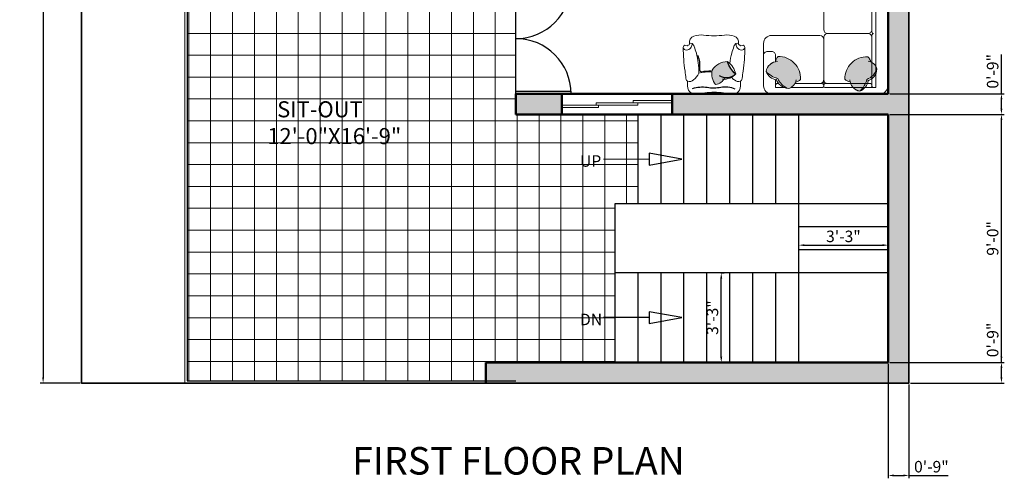
# Model space of a CAD drawing. Units: inches. Extents: x 1734 to 4011, y 1071 to 1891.
# Tile 10 of 27: x 2226 to 2654, y 1083 to 1282. Entities that reach past the tile are written whole.
import ezdxf

# ---------------------------------------------------------------- set-up
doc = ezdxf.new("R2010")
doc.units = ezdxf.units.IN
for name, color, linetype, lineweight in [('A-ANNO-DIMS', 2, 'Continuous', 18), ('A-ANNO-TEXT', 7, 'Continuous', 25), ('A-AREA-IDEN', 3, 'Continuous', 18), ('A-DOOR', 3, 'Continuous', 25), ('A-FLOR-OTLN', 7, 'Continuous', 25), ('A-FLOR-PATT', 252, 'Continuous', 13), ('A-FLOR-STRS', 2, 'Continuous', 25), ('A-FURN', 8, 'Continuous', 18), ('A-FURN-PATT', 252, 'Continuous', 13), ('A-GLAZ', 4, 'Continuous', 18), ('A-WALL', 7, 'Continuous', 50), ('A-WALL-PATT', 8, 'Continuous', 13), ('C-PROP', 1, 'Continuous', 35)]:
    doc.layers.add(name, color=color, linetype=linetype, lineweight=lineweight)
doc.layers.add('IFF-FURN-DETAIL', color=250, linetype='Continuous')
doc.styles.get("Standard").update_dxf_attribs({"font": 'arial.ttf'})
doc.dimstyles.new('ISO-25', dxfattribs={"dimtxt": 5, "dimasz": 2.5, "dimexe": 1.25, "dimexo": 0.625, "dimtad": 1, "dimdec": 1, "dimlunit": 3, "dimtxsty": 'Standard', "dimcen": 2.5, "dimclrt": 1, "dimadec": 0, "dimazin": 0, "dimtfac": 1, "dimtdec": 1, "dimtmove": 0, "dimatfit": 3, "dimfxl": 1, "dimarcsym": 0})

# ---------------------------------------------------------------- blocks, each defined once
blk = doc.blocks.new('*D17')
at = {"layer": 'A-ANNO-DIMS', "color": 0, "lineweight": -2, "transparency": 16777216}
for p, q in [((2251.86, 1844.06), (2234.55, 1844.06)), ((2235.8, 1841.56), (2235.8, 1126.56)), ((2251.86, 1124.06), (2234.55, 1124.06))]:
    blk.add_line(p, q, dxfattribs=at)
at = {"layer": 'A-ANNO-DIMS', "color": 0, "transparency": 16777216}
for points in [[(2235.38, 1841.56), (2236.21, 1841.56), (2235.8, 1844.06)], [(2235.38, 1126.56), (2236.21, 1126.56), (2235.8, 1124.06)]]:
    blk.add_solid(points, dxfattribs=at)
at = {"layer": 'Defpoints', "color": 0, "transparency": 16777216}
for p in [(2252.48, 1844.06), (2235.8, 1124.06), (2252.48, 1124.06)]:
    blk.add_point(p, dxfattribs=at)
at = {"layer": 'A-ANNO-DIMS', "color": 0, "transparency": 16777216, "insert": (2230.58, 1484.06), "char_height": 5, "attachment_point": 5, "rotation": 90}
blk.add_mtext("{\\H1.8x;60'}", dxfattribs=at)
blk = doc.blocks.new('*D18')
at = {"layer": 'A-ANNO-DIMS', "color": 0, "lineweight": -2, "transparency": 16777216}
for p, q in [((2530.68, 1172.06), (2532.08, 1172.06)), ((2530.83, 1135.56), (2530.83, 1169.56)), ((2530.68, 1133.06), (2532.08, 1133.06))]:
    blk.add_line(p, q, dxfattribs=at)
at = {"layer": 'A-ANNO-DIMS', "color": 0, "transparency": 16777216}
for points in [[(2530.41, 1169.56), (2531.25, 1169.56), (2530.83, 1172.06)], [(2530.41, 1135.56), (2531.25, 1135.56), (2530.83, 1133.06)]]:
    blk.add_solid(points, dxfattribs=at)
at = {"layer": 'Defpoints', "color": 0, "transparency": 16777216}
for p in [(2530.05, 1172.06), (2530.83, 1172.06), (2530.05, 1133.06)]:
    blk.add_point(p, dxfattribs=at)
at = {"layer": 'A-ANNO-DIMS', "color": 0, "transparency": 16777216, "insert": (2527.65, 1152.56), "char_height": 5, "attachment_point": 5, "rotation": 90}
blk.add_mtext('3\'-3"', dxfattribs=at)
blk = doc.blocks.new('*D19')
at = {"layer": 'A-ANNO-DIMS', "color": 0, "lineweight": -2, "transparency": 16777216}
for p, q in [((2564.48, 1186.44), (2564.48, 1182.86)), ((2566.98, 1184.11), (2600.98, 1184.11)), ((2603.48, 1186.44), (2603.48, 1182.86))]:
    blk.add_line(p, q, dxfattribs=at)
at = {"layer": 'A-ANNO-DIMS', "color": 0, "transparency": 16777216}
for points in [[(2566.98, 1184.52), (2566.98, 1183.69), (2564.48, 1184.11)], [(2600.98, 1184.52), (2600.98, 1183.69), (2603.48, 1184.11)]]:
    blk.add_solid(points, dxfattribs=at)
at = {"layer": 'Defpoints', "color": 0, "transparency": 16777216}
for p in [(2564.48, 1187.06), (2603.48, 1187.06), (2603.48, 1184.11)]:
    blk.add_point(p, dxfattribs=at)
at = {"layer": 'A-ANNO-DIMS', "color": 0, "transparency": 16777216, "insert": (2583.98, 1187.29), "char_height": 5, "attachment_point": 5}
blk.add_mtext('3\'-3"', dxfattribs=at)
blk = doc.blocks.new("MD D 4'")
for p, q in [((0, 24), (0, 0)), ((1, 24), (1, 0)), ((47, 24), (47, 0)), ((48, 24), (48, 0)), ((0, 0), (1, 0)), ((48, 0), (47, 0))]:
    blk.add_line(p, q)
for centre, start, end in [((0, 0), 0, 90), ((48, 0), 90, 180)]:
    blk.add_arc(centre, 24, start, end)
blk = doc.blocks.new('SOFA 1')
at = {"transparency": 33554687}
h = blk.add_hatch(color=256, dxfattribs=at)
h.dxf.hatch_style = 1
h.paths.add_polyline_path([(3723.52, 1308.63, 0.147724), (3717.76, 1305.24, 0.310469), (3722.42, 1300.4), (3722.42, 1300.25, 0.156703), (3723.62, 1297.8, 0.425821), (3734.69, 1309.08, 0.121928), (3732.05, 1310.63, 0.233216), (3728.6, 1313.59, 0.213835)])
h = blk.add_hatch(color=256, dxfattribs=at)
h.dxf.hatch_style = 1
h.paths.add_polyline_path([(3769.65, 1307.6, 0.084911), (3767.15, 1309.12, 0.046133), (3766.46, 1311.13), (3759.18, 1311.13, 0.039409), (3758.92, 1310.24, 0.165523), (3756.31, 1309.02, 0.42585), (3767.59, 1297.95, 0.121928), (3769.15, 1300.58, 0.027403), (3769.65, 1300.83)])
h.paths.add_polyline_path([(3765.34, 1313.08), (3760.4, 1313.08, 0.097704), (3759.18, 1311.13), (3766.46, 1311.13, 0.04873)])
h.paths.add_polyline_path([(3763.76, 1314.88, 0.16488), (3760.4, 1313.08), (3765.34, 1313.08, 0.051917)])
h.paths.add_polyline_path([(3771.6, 1305.17, 0.090388), (3769.65, 1307.6), (3769.65, 1300.83, 0.136035), (3771.6, 1302.77)])
h = blk.add_hatch(color=256, dxfattribs=at)
h.dxf.hatch_style = 1
h.paths.add_polyline_path([(3769.16, 1235.96, 0.122267), (3767.6, 1238.61, 0.425972), (3756.32, 1227.54, 0.165563), (3758.93, 1226.32, 0.309481), (3763.76, 1221.69, 0.002677), (3763.83, 1221.72, 0.146094), (3767.16, 1227.43, 0.212433), (3772.1, 1232.48, 0.235342)])
h = blk.add_hatch(color=256, dxfattribs=at)
h.dxf.hatch_style = 1
h.paths.add_polyline_path([(3769.16, 1225.36, 0.122267), (3767.6, 1228.01, 0.425972), (3756.32, 1216.94, 0.165563), (3758.93, 1215.72, 0.309481), (3763.76, 1211.09, 0.002677), (3763.83, 1211.12, 0.146094), (3767.16, 1216.83, 0.212433), (3772.1, 1221.88, 0.235342)])
for p, q in [((3720.45, 1316.13), (3773.58, 1316.13)), ((3777.51, 1312.19), (3777.51, 1213.72))]:
    blk.add_line(p, q, dxfattribs=at)
for points in [[(3717.76, 1305.24, -0.147724), (3723.52, 1308.63, -0.213355), (3728.59, 1313.59, 0.213355), (3723.52, 1308.63, 0.147724), (3717.76, 1305.24, -0.249545), (3722.86, 1309.34, 0.249545), (3717.75, 1305.25, 0.356779), (3723.4, 1300.28, -0.356779), (3717.76, 1305.24)], [(3728.58, 1313.6, -0.306333), (3732.42, 1309.31, 0.306333), (3728.58, 1313.6, 0.306674), (3722.72, 1308.89, -0.306674), (3728.58, 1313.6)], [(3763.76, 1314.88, -0.147724), (3767.15, 1309.12, -0.213355), (3772.1, 1304.05, 0.213355), (3767.15, 1309.12, 0.147724), (3763.76, 1314.88, -0.249545), (3767.86, 1309.77, 0.249545), (3763.77, 1314.89, 0.356779), (3758.8, 1309.23, -0.356779), (3763.76, 1314.88)], [(3734.69, 1309.08, -0.425972), (3723.62, 1297.8, -0.165552), (3722.4, 1300.4, 0.165552), (3723.62, 1297.79, 0.425972), (3734.69, 1309.07, 0.121514), (3732.07, 1310.63, -0.121514), (3734.69, 1309.08)], [(3767.6, 1297.95, -0.425972), (3756.31, 1309.01, -0.165552), (3758.92, 1310.24, 0.165552), (3756.31, 1309.02, 0.425972), (3767.59, 1297.95, 0.121514), (3769.14, 1300.57, -0.121514), (3767.6, 1297.95)], [(3772.11, 1304.06, -0.306333), (3767.83, 1300.22, 0.306333), (3772.11, 1304.06, 0.306674), (3767.4, 1309.91, -0.306674), (3772.11, 1304.06)], [(3770.44, 1286.63, -0.414214), (3769.66, 1287.4, 0.414214), (3770.44, 1286.63, 0.414214), (3769.66, 1285.83, -0.414214), (3770.44, 1286.63)], [(3748.01, 1262.99, -0.414214), (3746.05, 1264.95, 0.414214), (3748.01, 1262.97, 0.414213), (3746.05, 1261.01, -0.414213), (3748.01, 1262.99)], [(3770.44, 1262.99, -0.414214), (3769.66, 1263.77, 0.414214), (3770.44, 1262.99, 0.414214), (3769.66, 1262.19, -0.414214), (3770.44, 1262.99)], [(3770.83, 1262.97, -0.414214), (3771.61, 1262.19, 0.414214), (3770.83, 1262.99, 0.414214), (3771.61, 1263.77, -0.414214), (3770.83, 1262.97)], [(3748.01, 1239.35, -0.414214), (3746.05, 1241.31, 0.414214), (3748.01, 1239.33, 0.414213), (3746.05, 1237.37, -0.414213), (3748.01, 1239.35)], [(3767.7, 1239.33, -0.414214), (3769.66, 1237.37, 0.414214), (3767.7, 1239.35, 0.414214), (3769.66, 1241.31, -0.414214), (3767.7, 1239.33)], [(3756.32, 1227.54, -0.425972), (3767.6, 1238.61, -0.121514), (3769.16, 1235.98, 0.121514), (3767.6, 1238.61, 0.425972), (3756.32, 1227.54, 0.165552), (3758.93, 1226.32, -0.165552), (3756.32, 1227.54)], [(3772.1, 1232.5, -0.306674), (3767.41, 1226.64, 0.306674), (3772.1, 1232.5, 0.306333), (3767.84, 1236.34, -0.306333), (3772.1, 1232.5)], [(3770.44, 1239.35, -0.414214), (3769.66, 1240.13, 0.414214), (3770.44, 1239.33, 0.414214), (3769.66, 1238.55, -0.414214), (3770.44, 1239.35)], [(3770.83, 1239.33, -0.414214), (3771.61, 1238.55, 0.414214), (3770.83, 1239.35, 0.414214), (3771.61, 1240.13, -0.414214), (3770.83, 1239.33)], [(3763.78, 1221.67, 0.249545), (3767.87, 1226.78, -0.249545), (3763.76, 1221.69, -0.356779), (3758.81, 1227.32, 0.356779), (3763.77, 1221.68, 0.147724), (3767.16, 1227.43, 0.213355), (3772.11, 1232.51, -0.213355), (3767.16, 1227.43, -0.147724), (3763.78, 1221.67)], [(3756.32, 1216.94, -0.200233), (3759.49, 1224.76, 0.200233), (3756.32, 1216.94, 0.165552), (3758.93, 1215.72, -0.165552), (3756.32, 1216.94)], [(3772.1, 1221.9, -0.306674), (3767.41, 1216.04, 0.306674), (3772.1, 1221.9, -0.213355), (3767.16, 1216.83, -0.147724), (3763.77, 1211.08, 0.147724), (3767.15, 1216.83, 0.213355), (3772.1, 1221.9)], [(3763.76, 1211.09, -0.356779), (3758.81, 1216.72, 0.356779), (3763.76, 1211.09, 0.249545), (3767.87, 1216.18, -0.249545), (3763.76, 1211.09)]]:
    blk.add_lwpolyline(points, format="xyb", dxfattribs=at)
for points in [[(3722.42, 1313.08), (3722.42, 1309.23), (3722.42, 1313.08), (3726.57, 1313.08)], [(3729.85, 1313.08), (3745.25, 1313.08)], [(3768.11, 1313.08), (3746.78, 1313.08)], [(3771.6, 1313.08), (3767.75, 1313.08), (3771.6, 1313.08), (3771.6, 1308.93)], [(3771.6, 1313.08), (3771.61, 1233.74)], [(3716.51, 1312.2), (3716.51, 1291.44)], [(3723.21, 1311.13), (3723.93, 1311.13)], [(3731.82, 1311.13), (3745.25, 1311.13)], [(3746.01, 1312.3), (3746.01, 1288.55)], [(3746.01, 1310.97), (3746.01, 1311.36)], [(3746.01, 1288.54), (3746.01, 1308.23)], [(3768.87, 1311.13), (3746.78, 1311.13)], [(3769.66, 1287.39), (3769.65, 1312.3)], [(3769.65, 1309.43), (3769.65, 1308.71)], [(3722.42, 1300.39), (3722.42, 1297.33)], [(3720.45, 1295.38), (3718.48, 1295.38)], [(3720.45, 1287.5), (3744.09, 1287.5)], [(3746.02, 1284.63), (3746.02, 1264.94)], [(3747.99, 1286.6), (3767.69, 1286.6)], [(3769.66, 1263.75), (3769.66, 1285.81)], [(3769.66, 1277.18), (3769.66, 1263.75)], [(3746.02, 1260.99), (3746.02, 1241.3)], [(3747.99, 1262.97), (3767.69, 1262.97)], [(3769.66, 1240.12), (3769.66, 1262.18)], [(3770.43, 1262.97), (3770.82, 1262.97)], [(3746.02, 1237.36), (3746.02, 1213.74)], [(3747.99, 1239.33), (3767.69, 1239.33)], [(3769.66, 1235.71), (3769.66, 1238.54)], [(3770.43, 1239.33), (3770.82, 1239.33)], [(3769.66, 1225.11), (3769.66, 1227.82)], [(3771.61, 1223.14), (3771.61, 1230.47)], [(3767.76, 1215.72), (3771.61, 1215.72), (3771.61, 1219.84), (3771.61, 1215.72)], [(3769.66, 1216.5), (3769.66, 1217.22)], [(3753.91, 1211.77), (3753.91, 1213.74)], [(3755.86, 1215.72), (3758.92, 1215.72)], [(3749.97, 1209.8), (3773.58, 1209.8)]]:
    blk.add_lwpolyline(points, close=True, dxfattribs=at)
for points in [[(3770.43, 1313.08, 0.414214), (3769.65, 1312.3, -0.414214)], [(3771.6, 1312.3, 0.414214), (3770.82, 1313.08, -0.414214)], [(3722.42, 1311.91, 0.414214), (3723.2, 1311.13, -0.414214)], [(3716.51, 1297.34, 0.414214), (3718.47, 1295.38, -0.414214)], [(3720.44, 1295.38, 0.414214), (3722.4, 1297.34, -0.414214)], [(3716.51, 1291.45, 0.414212), (3720.44, 1287.52, -0.414212)], [(3746.03, 1288.56, 0.414214), (3747.99, 1286.6, 0.414213), (3746.03, 1284.64, -0.414213), (3747.99, 1286.6, -0.414214)], [(3769.66, 1284.64, 0.414214), (3767.7, 1286.6, 0.414214), (3769.66, 1288.56, -0.414214), (3767.7, 1286.6, -0.414214)], [(3769.66, 1261.01, 0.414214), (3767.7, 1262.97, 0.414214), (3769.66, 1264.93, -0.414214), (3767.7, 1262.97, -0.414214)], [(3769.16, 1225.36, 0.071861), (3768.39, 1227.01, -0.071861)], [(3772.13, 1221.9, 0.306333), (3767.84, 1225.74, -0.306333)], [(3769.66, 1216.52, 0.414214), (3770.44, 1215.74, -0.414214)], [(3770.83, 1215.74, 0.414214), (3771.61, 1216.52, -0.414214)], [(3746.05, 1213.76, 0.414212), (3749.98, 1209.82, -0.414212)], [(3755.87, 1215.72, 0.414214), (3753.91, 1213.76, -0.414214)], [(3755.87, 1209.8, -0.414214), (3753.91, 1211.76, 0.414214)]]:
    blk.add_lwpolyline(points, format="xyb", close=True, dxfattribs=at)
for centre, radius, start, end in [((3720.44, 1312.2), 3.93, 90.0002, 179.9998), ((3720.44, 1312.19), 3.94, 89.9158, 179.9154), ((3745.22, 1312.29), 0.789, 0.8425, 90.8425), ((3746.8, 1312.29), 0.789, 89.1575, 179.1575), ((3768.87, 1312.3), 0.777, 360, 90), ((3773.58, 1312.2), 3.93, 0.0002, 89.9998), ((3773.57, 1312.19), 3.94, 359.9158, 89.9154), ((3744.09, 1309.21), 1.92, 358.766, 90.5111), ((3745.24, 1311.91), 0.777, 270, 0), ((3745.24, 1311.91), 0.777, 270, 0), ((3746.79, 1311.91), 0.777, 180, 270), ((3746.79, 1311.91), 0.777, 180, 270), ((3747.93, 1309.21), 1.92, 89.4889, 181.234), ((3768.87, 1311.91), 0.777, 270, 0), ((3744.08, 1289.48), 1.96, 270, 360), ((3744.08, 1289.48), 1.96, 270, 360), ((3773.58, 1213.73), 3.93, 270.0002, 359.9998), ((3773.59, 1213.73), 3.93, 269.9156, 359.9152)]:
    blk.add_arc(centre, radius, start, end, dxfattribs=at)
blk = doc.blocks.new('PILLOW-1')
at = {"color": 0}
blk.add_lwpolyline([(198, -165, -0.232884), (126, -346, -0.184752), (-44, -234, -0.286563), (75, -22, -0.237978), (273, -68, -0.243587), (179, -195, 4.263709)], format="xyb", dxfattribs=at)
at = {"layer": 'IFF-FURN-DETAIL'}
blk.add_lwpolyline([(148, -118, -0.343333), (126, -342, 0.126408), (-40, -233, -5.969376)], format="xyb", dxfattribs=at)
blk = doc.blocks.new('CLNG90')
for points in [[(689, 370, 0.157831), (677, 385, 0.121013), (646, 395, -0.017334), (547, 407, 0.041496), (215, 431, 0.153531), (191, 423, 0.382906), (185, 395, -0.284047), (184, 361, 0.011997), (177, 351, -0.370479), (160, 345, 0.380647), (56, 282, 0.117468), (41, 146, -0.027775), (50, 0, -8.773898)], [(160, 345, 0.22481), (160, 306, 0.055398), (209, 322, 0.180116), (249, 368, 0.194833), (248, 405, 0.242377), (215, 431, 1.52074)], [(160, 345, 0.22481), (160, 306, 0.055398), (209, 322, 0.180116), (249, 368, 0.194833), (248, 405, 0.242377), (215, 431, 1.52074)], [(689, 370, -0.235486), (671, 286, -0.134038), (574, 215, -0.079303), (293, 248, -0.027048), (199, 280, -0.106276), (160, 306, -1.699)], [(689, 370, -0.235486), (671, 286, -0.134038), (574, 215, -0.079303), (293, 248, -0.027048), (199, 280, -0.106276), (160, 306, -1.699)], [(689, 370, -0.146607), (814, 357, -0.305296), (862, 286, -0.042137), (852, 131, 0.040285), (843, 0, 3.952121)], [(574, 215, 0.061244), (556, 29, 3.376255)], [(574, 215, 0.061244), (556, 29, 3.376255)], [(689, -370, -0.157831), (677, -385, -0.121013), (646, -395, 0.017334), (547, -407, -0.041496), (215, -431, -0.153531), (191, -423, -0.382906), (185, -395, 0.284047), (184, -361, -0.011997), (177, -351, 0.370479), (160, -345, -0.380647), (56, -282, -0.117468), (41, -146, 0.027775), (50, 0, 8.773898)], [(689, -370, 0.146607), (814, -357, 0.305296), (862, -286, 0.042137), (852, -131, -0.040285), (843, 0, -3.952121)], [(437, -220, 0.041086), (293, -248, 0.027048), (199, -280, 0.106276), (160, -306, 1.699)], [(437, -220, 0.041086), (293, -248, 0.027048), (199, -280, 0.106276), (160, -306, 1.699)], [(689, -370, 0.235486), (671, -286, 0.060693), (632, -247, 0.001296)], [(689, -370, 0.235486), (671, -286, 0.060693), (632, -247, 0.001296)], [(160, -345, -0.22481), (160, -306, -0.055398), (209, -322, -0.180116), (249, -368, -0.194833), (248, -405, -0.242377), (215, -431, -1.52074)], [(160, -345, -0.22481), (160, -306, -0.055398), (209, -322, -0.180116), (249, -368, -0.194833), (248, -405, -0.242377), (215, -431, -1.52074)]]:
    blk.add_lwpolyline(points, format="xyb")
at = {"layer": 'IFF-FURN-DETAIL'}
for points in [[(791, 301, 0.124986), (774, 96, -0.091334), (771, -95, 0.164688), (797, -292, 1.068868)], [(791, 301, 0.124986), (774, 96, -0.091334), (771, -95, 0.164688), (797, -292, 1.068868)], [(328, 228, 0.109125), (508, 203, -0.16587), (546, 194, -0.314359), (555, 172, 0.072017), (544, 42, 4.351186)], [(328, 228, 0.109125), (508, 203, -0.16587), (546, 194, -0.314359), (555, 172, 0.072017), (544, 42, 4.351186)]]:
    blk.add_lwpolyline(points, format="xyb", dxfattribs=at)
at = {"xscale": 1.016, "yscale": 1.016, "zscale": 1.016}
blk.add_blockref('PILLOW-1', (458, 47), dxfattribs=at)
blk.add_blockref('PILLOW-1', (458, 47), dxfattribs=at)
blk = doc.blocks.new('*D115')
at = {"layer": 'A-ANNO-DIMS', "color": 0, "lineweight": -2, "transparency": 16777216}
for p, q in [((2652.73, 1133.06), (2652.73, 1150.1)), ((2604.11, 1133.06), (2653.98, 1133.06)), ((2652.73, 1126.56), (2652.73, 1130.56)), ((2613.11, 1124.06), (2653.98, 1124.06))]:
    blk.add_line(p, q, dxfattribs=at)
at = {"layer": 'A-ANNO-DIMS', "color": 0, "transparency": 16777216}
for points in [[(2652.31, 1130.56), (2653.15, 1130.56), (2652.73, 1133.06)], [(2652.31, 1126.56), (2653.15, 1126.56), (2652.73, 1124.06)]]:
    blk.add_solid(points, dxfattribs=at)
at = {"layer": 'Defpoints', "color": 0, "transparency": 16777216}
for p in [(2603.48, 1133.06), (2652.73, 1133.06), (2612.48, 1124.06)]:
    blk.add_point(p, dxfattribs=at)
at = {"layer": 'A-ANNO-DIMS', "color": 1, "transparency": 16777216, "insert": (2649.55, 1142.83), "char_height": 5, "attachment_point": 5, "rotation": 90}
blk.add_mtext('0\'-9"', dxfattribs=at)
blk = doc.blocks.new('*D116')
at = {"layer": 'A-ANNO-DIMS', "color": 0, "lineweight": -2, "transparency": 16777216}
for p, q in [((2604.11, 1241.06), (2653.98, 1241.06)), ((2652.73, 1135.56), (2652.73, 1238.56)), ((2604.11, 1133.06), (2653.98, 1133.06))]:
    blk.add_line(p, q, dxfattribs=at)
at = {"layer": 'A-ANNO-DIMS', "color": 0, "transparency": 16777216}
for points in [[(2652.31, 1238.56), (2653.15, 1238.56), (2652.73, 1241.06)], [(2652.31, 1135.56), (2653.15, 1135.56), (2652.73, 1133.06)]]:
    blk.add_solid(points, dxfattribs=at)
at = {"layer": 'Defpoints', "color": 0, "transparency": 16777216}
for p in [(2603.48, 1241.06), (2652.73, 1241.06), (2603.48, 1133.06)]:
    blk.add_point(p, dxfattribs=at)
at = {"layer": 'A-ANNO-DIMS', "color": 1, "transparency": 16777216, "insert": (2649.55, 1187.06), "char_height": 5, "attachment_point": 5, "rotation": 90}
blk.add_mtext('9\'-0"', dxfattribs=at)
blk = doc.blocks.new('*D117')
at = {"layer": 'A-ANNO-DIMS', "color": 0, "lineweight": -2, "transparency": 16777216}
for p, q in [((2652.73, 1250.06), (2652.73, 1267.1)), ((2604.11, 1250.06), (2653.98, 1250.06)), ((2652.73, 1243.56), (2652.73, 1247.56)), ((2604.11, 1241.06), (2653.98, 1241.06))]:
    blk.add_line(p, q, dxfattribs=at)
at = {"layer": 'A-ANNO-DIMS', "color": 0, "transparency": 16777216}
for points in [[(2652.31, 1247.56), (2653.15, 1247.56), (2652.73, 1250.06)], [(2652.31, 1243.56), (2653.15, 1243.56), (2652.73, 1241.06)]]:
    blk.add_solid(points, dxfattribs=at)
at = {"layer": 'Defpoints', "color": 0, "transparency": 16777216}
for p in [(2603.48, 1250.06), (2652.73, 1250.06), (2603.48, 1241.06)]:
    blk.add_point(p, dxfattribs=at)
at = {"layer": 'A-ANNO-DIMS', "color": 1, "transparency": 16777216, "insert": (2649.55, 1259.83), "char_height": 5, "attachment_point": 5, "rotation": 90}
blk.add_mtext('0\'-9"', dxfattribs=at)
blk = doc.blocks.new('*D118')
at = {"layer": 'A-ANNO-DIMS', "color": 0, "lineweight": -2, "transparency": 16777216}
for p, q in [((2603.48, 1132.44), (2603.48, 1082.56)), ((2612.48, 1123.44), (2612.48, 1082.56)), ((2605.98, 1083.81), (2609.98, 1083.81)), ((2612.48, 1083.81), (2629.52, 1083.81))]:
    blk.add_line(p, q, dxfattribs=at)
at = {"layer": 'A-ANNO-DIMS', "color": 0, "transparency": 16777216}
for points in [[(2605.98, 1084.23), (2605.98, 1083.39), (2603.48, 1083.81)], [(2609.98, 1084.23), (2609.98, 1083.39), (2612.48, 1083.81)]]:
    blk.add_solid(points, dxfattribs=at)
at = {"layer": 'Defpoints', "color": 0, "transparency": 16777216}
for p in [(2603.48, 1133.06), (2612.48, 1124.06), (2612.48, 1083.81)]:
    blk.add_point(p, dxfattribs=at)
at = {"layer": 'A-ANNO-DIMS', "color": 1, "transparency": 16777216, "insert": (2622.25, 1086.99), "char_height": 5, "attachment_point": 5}
blk.add_mtext('0\'-9"', dxfattribs=at)

msp = doc.modelspace()

# ---------------------------------------------------------------- hatches: boundary and pattern name
at = {"layer": 'A-FLOR-PATT'}
h = msp.add_hatch(dxfattribs=at)
h.set_pattern_fill('ANSI37', color=256, scale=3, angle=45)
h.set_pattern_definition([(90, (-758.361, 0), (-9.525, 0), []), (180, (-758.361, 0), (-9e-16, -9.525), [])])
h.paths.add_polyline_path([(2441.48, 1241.06), (2441.48, 1325.06), (2298.48, 1325.06), (2298.48, 1125.06), (2428.48, 1125.06), (2428.48, 1133.06), (2484.48, 1133.06), (2484.48, 1202.06), (2494.48, 1202.06), (2494.48, 1241.06)])
h.paths.add_polyline_path([(2467.59, 1146.53), (2480.18, 1146.53), (2480.18, 1156.83), (2467.59, 1156.83)], flags=24)
h.paths.add_polyline_path([(2467.58, 1215.53), (2479.78, 1215.53), (2479.78, 1225.83), (2467.58, 1225.83)], flags=24)
h.paths.add_polyline_path([(2330.54, 1224.14), (2390.38, 1224.14), (2390.38, 1250.26), (2330.54, 1250.26)], flags=24)
at = {"layer": 'A-FURN-PATT'}
h = msp.add_hatch(dxfattribs=at)
h.set_pattern_fill('ANSI32', color=256)
h.set_pattern_definition([(45, (-758.361, 0), (-6.735192, 6.735192), []), (45, (-753.871, 0), (-6.735192, 6.735192), [])])
h.paths.add_polyline_path([(2366.48, 1466.06), (2306.48, 1466.06), (2306.48, 1448.06), (2366.48, 1448.06)])
h.paths.add_polyline_path([(2310.37, 1452.28), (2359.82, 1452.28), (2359.82, 1462.58), (2310.37, 1462.58)], flags=24)
h.paths.add_polyline_path([(2525.12, 1646.17), (2525.12, 1700.88), (2499, 1700.88), (2499, 1646.17)], flags=9)
h.paths.add_polyline_path([(2555.1, 1646.17), (2555.1, 1700.88), (2528.98, 1700.88), (2528.98, 1646.17)], flags=9)
h.paths.add_polyline_path([(2492.08, 1807.82), (2546.48, 1807.82), (2546.48, 1833.94), (2492.08, 1833.94)], flags=9)
h.paths.add_polyline_path([(2464.41, 1783), (2507.08, 1783), (2507.08, 1791.24), (2464.41, 1791.24)], flags=9)
h.paths.add_polyline_path([(2467.59, 1146.53), (2480.18, 1146.53), (2480.18, 1156.83), (2467.59, 1156.83)], flags=9)
h.paths.add_polyline_path([(2467.58, 1215.53), (2479.78, 1215.53), (2479.78, 1225.83), (2467.58, 1225.83)], flags=9)
h.paths.add_polyline_path([(2292.19, 1646.17), (2292.19, 1700.88), (2266.07, 1700.88), (2266.07, 1646.17)], flags=9)
h.paths.add_polyline_path([(2504.62, 1567.64), (2559.02, 1567.64), (2559.02, 1593.76), (2504.62, 1593.76)], flags=9)
h.paths.add_polyline_path([(2562.71, 1614.15), (2583.08, 1614.15), (2583.08, 1624.45), (2562.71, 1624.45)], flags=9)
h.paths.add_polyline_path([(2522.41, 1650.28), (2571.86, 1650.28), (2571.86, 1660.58), (2522.41, 1660.58)], flags=9)
h.paths.add_polyline_path([(2504.36, 1707.67), (2564.2, 1707.67), (2564.2, 1733.79), (2504.36, 1733.79)], flags=9)
h.paths.add_polyline_path([(2381.34, 1790.51), (2430.31, 1790.51), (2430.31, 1816.63), (2381.34, 1816.63)], flags=9)
h.paths.add_polyline_path([(2291.99, 1790.51), (2340.95, 1790.51), (2340.95, 1816.63), (2291.99, 1816.63)], flags=9)
h.paths.add_polyline_path([(2330.54, 1224.14), (2390.38, 1224.14), (2390.38, 1250.26), (2330.54, 1250.26)], flags=9)
h.paths.add_polyline_path([(2425.61, 1508.95), (2480.02, 1508.95), (2480.02, 1535.07), (2425.61, 1535.07)], flags=9)
h.paths.add_polyline_path([(2505.48, 1357.1), (2574.53, 1357.1), (2574.53, 1383.22), (2505.48, 1383.22)], flags=9)
h.paths.add_polyline_path([(2530.46, 1484.55), (2584.86, 1484.55), (2584.86, 1510.67), (2530.46, 1510.67)], flags=9)
h.paths.add_polyline_path([(2349.79, 1659.95), (2415.08, 1659.95), (2415.08, 1686.07), (2349.79, 1686.07)], flags=9)
h = msp.add_hatch(color=256, dxfattribs=at)
h.dxf.hatch_style = 1
h.paths.add_polyline_path([(2526.92, 1260.29, 0.237978), (2528.37, 1254.06, 0.250405), (2532.44, 1257.12, 0.218011), (2537, 1258.66, -0.129718), (2533.5, 1264.05, 0.283254)])
at = {"layer": 'A-WALL-PATT'}
h = msp.add_hatch(color=256, dxfattribs=at)
h.dxf.hatch_style = 1
h.paths.add_polyline_path([(2612.48, 1844.06), (2261.48, 1844.06), (2261.48, 1758.06), (2270.05, 1758.06), (2270.05, 1763.06), (2266.48, 1763.06), (2266.48, 1835.06), (2353.48, 1835.06), (2353.48, 1793.06), (2358.48, 1793.06), (2358.48, 1835.06), (2445.48, 1835.06), (2445.48, 1763.06), (2393.48, 1763.06), (2393.48, 1758.06), (2445.48, 1758.06), (2445.48, 1617.06), (2450.48, 1617.06), (2450.48, 1641.06), (2454.48, 1641.06), (2454.48, 1646.06), (2450.48, 1646.06), (2450.48, 1790.06), (2456.52, 1790.06), (2456.52, 1799.06), (2450.48, 1799.06), (2450.48, 1839.06), (2603.48, 1839.06), (2603.48, 1799.06), (2585.48, 1799.06), (2585.48, 1790.06), (2603.48, 1790.06), (2603.48, 1646.06), (2490.48, 1646.06), (2490.48, 1641.06), (2603.48, 1641.06), (2603.48, 1601.06), (2555.48, 1601.06), (2555.48, 1598.06), (2603.48, 1598.06), (2603.48, 1530.06), (2588.98, 1530.06), (2588.98, 1525.06), (2603.48, 1525.06), (2603.48, 1471.06), (2582.98, 1471.06), (2582.98, 1466.06), (2612.48, 1466.06)])
h.paths.add_polyline_path([(2612.48, 1466.06), (2603.48, 1466.06), (2603.48, 1250.06), (2509.48, 1250.06), (2509.48, 1241.06), (2603.48, 1241.06), (2603.48, 1133.06), (2428.48, 1133.06), (2428.48, 1124.06), (2612.48, 1124.06)])
h = msp.add_hatch(color=256, dxfattribs=at)
h.dxf.hatch_style = 1
h.paths.add_polyline_path([(2306.48, 1543.06), (2297.48, 1543.06), (2297.48, 1364.06), (2306.48, 1364.06), (2306.48, 1466.06), (2400.48, 1466.06), (2400.48, 1471.06), (2371.48, 1471.06), (2371.48, 1483.06), (2366.48, 1483.06), (2366.48, 1471.06), (2306.48, 1471.06)])
h.paths.add_polyline_path([(2348.98, 1334.06), (2297.48, 1334.06), (2297.48, 1325.06), (2348.98, 1325.06)])
h.paths.add_polyline_path([(2450.48, 1466.06), (2455.48, 1466.06), (2455.48, 1471.06), (2436.48, 1471.06), (2436.48, 1466.06), (2445.48, 1466.06), (2445.48, 1334.06), (2402.98, 1334.06), (2402.98, 1325.06), (2450.48, 1325.06)])
h.paths.add_polyline_path([(2450.48, 1301.06), (2441.48, 1301.06), (2441.48, 1298.06), (2450.48, 1298.06)])
h.paths.add_polyline_path([(2450.48, 1581.06), (2445.48, 1581.06), (2445.48, 1577.06), (2302.48, 1577.06), (2302.48, 1582.06), (2297.48, 1582.06), (2297.48, 1567.06), (2306.48, 1567.06), (2306.48, 1572.06), (2366.48, 1572.06), (2366.48, 1513.06), (2371.48, 1513.06), (2371.48, 1572.06), (2450.48, 1572.06)])
h.paths.add_polyline_path([(2302.48, 1636.07), (2297.48, 1636.07), (2297.48, 1612.06), (2302.48, 1612.06)])
h.paths.add_polyline_path([(2363.48, 1763.06), (2294.05, 1763.06), (2294.05, 1758.06), (2297.48, 1758.06), (2297.48, 1684.07), (2302.48, 1684.07), (2302.48, 1758.06), (2363.48, 1758.06)])
h.paths.add_polyline_path([(2461.48, 1250.06), (2441.48, 1250.06), (2441.48, 1241.06), (2461.48, 1241.06)])

# ---------------------------------------------------------------- linework, layer by layer
at = {"layer": 'A-FLOR-OTLN'}
msp.add_lwpolyline([(2441.48, 1241.06), (2441.48, 1325.06), (2298.48, 1325.06), (2298.48, 1125.06), (2441.48, 1125.06)], dxfattribs=at)
at = {"layer": 'A-FLOR-STRS'}
for p, q in [((2494.48, 1241.06), (2494.48, 1202.06)), ((2504.48, 1241.06), (2504.48, 1202.06)), ((2514.48, 1241.06), (2514.48, 1202.06)), ((2524.48, 1241.06), (2524.48, 1202.06)), ((2534.48, 1241.06), (2534.48, 1202.06)), ((2544.48, 1241.06), (2544.48, 1202.06)), ((2554.48, 1241.06), (2554.48, 1202.06)), ((2564.48, 1241.06), (2564.48, 1133.06)), ((2603.48, 1202.06), (2484.48, 1202.06)), ((2484.48, 1202.06), (2484.48, 1133.06)), ((2603.48, 1192.06), (2564.48, 1192.06)), ((2603.48, 1182.06), (2564.48, 1182.06)), ((2603.48, 1172.06), (2484.48, 1172.06)), ((2494.48, 1172.06), (2494.48, 1133.06)), ((2504.48, 1172.06), (2504.48, 1133.06)), ((2514.48, 1172.06), (2514.48, 1133.06)), ((2524.48, 1172.06), (2524.48, 1133.06)), ((2534.48, 1172.06), (2534.48, 1133.06)), ((2544.48, 1172.06), (2544.48, 1133.06)), ((2554.48, 1172.06), (2554.48, 1133.06)), ((2499.48, 1152.56), (2479.56, 1152.56))]:
    msp.add_line(p, q, dxfattribs=at)
for points in [[(2513.64, 1221.56), (2499.48, 1224.11), (2499.48, 1219.01)], [(2513.64, 1152.56), (2499.48, 1155.11), (2499.48, 1150.01)]]:
    msp.add_lwpolyline(points, close=True, dxfattribs=at)
at = {"layer": 'A-FURN'}
for p, q in [((2297.48, 1124.06), (2297.48, 1582.06)), ((2298.48, 1125.06), (2298.48, 1325.06)), ((2499.48, 1221.56), (2479.56, 1221.56)), ((2298.48, 1125.06), (2428.48, 1125.06))]:
    msp.add_line(p, q, dxfattribs=at)
at = {"layer": 'A-GLAZ'}
for p, q in [((2492.48, 1247.06), (2509.48, 1247.06)), ((2492.48, 1246.06), (2492.48, 1247.06)), ((2461.48, 1245.06), (2494.48, 1245.06)), ((2461.48, 1244.06), (2477.48, 1244.06)), ((2476.48, 1246.06), (2509.48, 1246.06)), ((2476.48, 1245.06), (2476.48, 1246.06)), ((2477.48, 1244.06), (2477.48, 1245.06)), ((2494.48, 1245.06), (2494.48, 1246.06))]:
    msp.add_line(p, q, dxfattribs=at)
at = {"layer": 'A-WALL'}
for p, q in [((2603.48, 1466.06), (2603.48, 1250.06)), ((2441.48, 1250.06), (2441.48, 1241.06)), ((2603.48, 1250.06), (2441.48, 1250.06)), ((2461.48, 1250.06), (2461.48, 1241.06)), ((2509.48, 1250.06), (2509.48, 1241.06)), ((2603.48, 1241.06), (2441.48, 1241.06)), ((2603.48, 1241.06), (2603.48, 1133.06)), ((2428.48, 1133.06), (2428.48, 1124.06)), ((2603.48, 1133.06), (2428.48, 1133.06))]:
    msp.add_line(p, q, dxfattribs=at)
at = {"layer": 'C-PROP'}
msp.add_lwpolyline([(2428.48, 1124.06), (2252.48, 1124.06), (2252.48, 1844.06), (2612.48, 1844.06), (2612.48, 1124.06), (2428.48, 1124.06)], dxfattribs=at)

# ---------------------------------------------------------------- block references
at = {"layer": 'A-DOOR', "rotation": 270}
msp.add_blockref("MD D 4'", (2441.48, 1298.06), dxfattribs=at)
at = {"layer": 'A-FURN'}
for name, p, xscale, yscale, zscale, rotation in [('SOFA 1', (-749.74, 2418.33), -0.887653230693335, 0.887653230693335, 0.887653230693335, 180), ('CLNG90', (2527.69, 1276.85), -0.031001591544, 0.031001591544, 0.031001591544, 90)]:
    msp.add_blockref(name, p, dxfattribs=dict(at, xscale=xscale, yscale=yscale, zscale=zscale, rotation=rotation))

# ---------------------------------------------------------------- texts
at = {"layer": 'A-ANNO-TEXT', "attachment_point": 1}
for s, width, insert, char_height in [('UP', 10.7355, (2469.38, 1223.26), 5), ('DN', 10.7355, (2469.38, 1154.26), 5), ('FIRST FLOOR PLAN', 228.5661, (2370.24, 1096.19), 12)]:
    msp.add_mtext_dynamic_manual_height_columns(s, width=width, gutter_width=12.5, heights=[0], dxfattribs=dict(at, insert=insert, char_height=char_height))
at = {"layer": 'A-AREA-IDEN', "insert": (2333.35, 1246.78), "char_height": 7, "attachment_point": 1}
msp.add_mtext_dynamic_manual_height_columns('  SIT-OUT\\P12\'-0"X16\'-9"', width=86.9528, gutter_width=12.5, heights=[0], dxfattribs=at)

# ---------------------------------------------------------------- dimensions: what is measured, and where the dimension line sits
at = {"layer": 'A-ANNO-DIMS'}
dim = msp.add_linear_dim(base=(2235.8, 1124.06), p1=(2252.48, 1844.06), p2=(2252.48, 1124.06), angle=90, text='{\\H1.8x;<>}', dimstyle='ISO-25', override={"dimclrd": 0, "dimclre": 0, "dimclrt": 0}, dxfattribs=at)
dim.commit()
dim.dimension.update_dxf_attribs({"geometry": '*D17', "text_midpoint": (2230.58, 1484.06)})
for base, p1, p2, override, picture, middle in [((2652.73, 1250.06), (2603.48, 1241.06), (2603.48, 1250.06), {"dimdec": 1, "dimlfac": 1, "dimrnd": 0, "dimzin": 1, "dimdsep": 46, "dimlunit": 4, "dimfrac": 2}, '*D117', (2649.55, 1259.83)), ((2652.73, 1241.06), (2603.48, 1133.06), (2603.48, 1241.06), {"dimdec": 1, "dimlfac": 1, "dimrnd": 0, "dimzin": 1, "dimdsep": 46, "dimlunit": 4, "dimfrac": 2}, '*D116', (2649.55, 1187.06)), ((2530.83, 1172.06), (2530.05, 1133.06), (2530.05, 1172.06), {"dimclrd": 0, "dimclre": 0, "dimclrt": 0}, '*D18', (2527.65, 1152.56)), ((2652.73, 1133.06), (2612.48, 1124.06), (2603.48, 1133.06), {"dimdec": 1, "dimlfac": 1, "dimrnd": 0, "dimzin": 1, "dimdsep": 46, "dimlunit": 4, "dimfrac": 2}, '*D115', (2649.55, 1142.83))]:
    dim = msp.add_linear_dim(base=base, p1=p1, p2=p2, angle=90, dimstyle='ISO-25', override=override, dxfattribs=at)
    dim.commit()
    dim.dimension.update_dxf_attribs({"geometry": picture, "text_midpoint": middle})
for base, p1, p2, override, picture, middle in [((2603.48, 1184.11), (2564.48, 1187.06), (2603.48, 1187.06), {"dimclrd": 0, "dimclre": 0, "dimclrt": 0}, '*D19', (2583.98, 1187.29)), ((2612.48, 1083.81), (2603.48, 1133.06), (2612.48, 1124.06), {"dimdec": 1, "dimlfac": 1, "dimrnd": 0, "dimzin": 1, "dimdsep": 46, "dimlunit": 4, "dimfrac": 2}, '*D118', (2622.25, 1086.99))]:
    dim = msp.add_linear_dim(base=base, p1=p1, p2=p2, dimstyle='ISO-25', override=override, dxfattribs=at)
    dim.commit()
    dim.dimension.update_dxf_attribs({"geometry": picture, "text_midpoint": middle})

doc.saveas('drawing.dxf')
